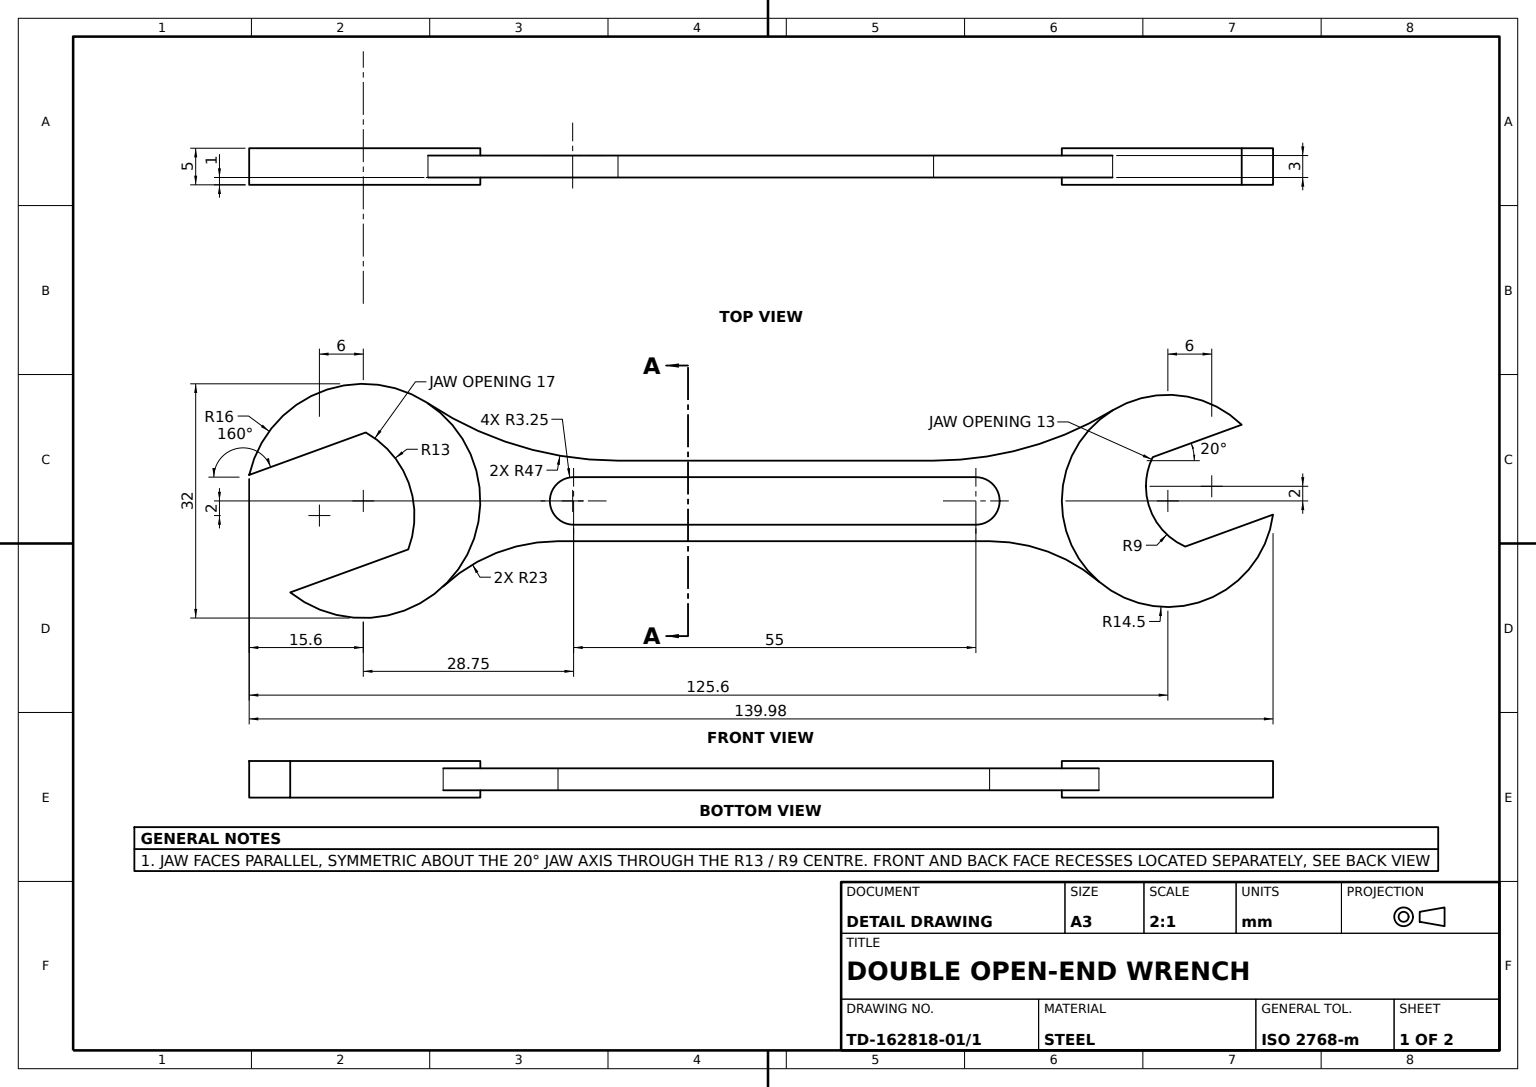
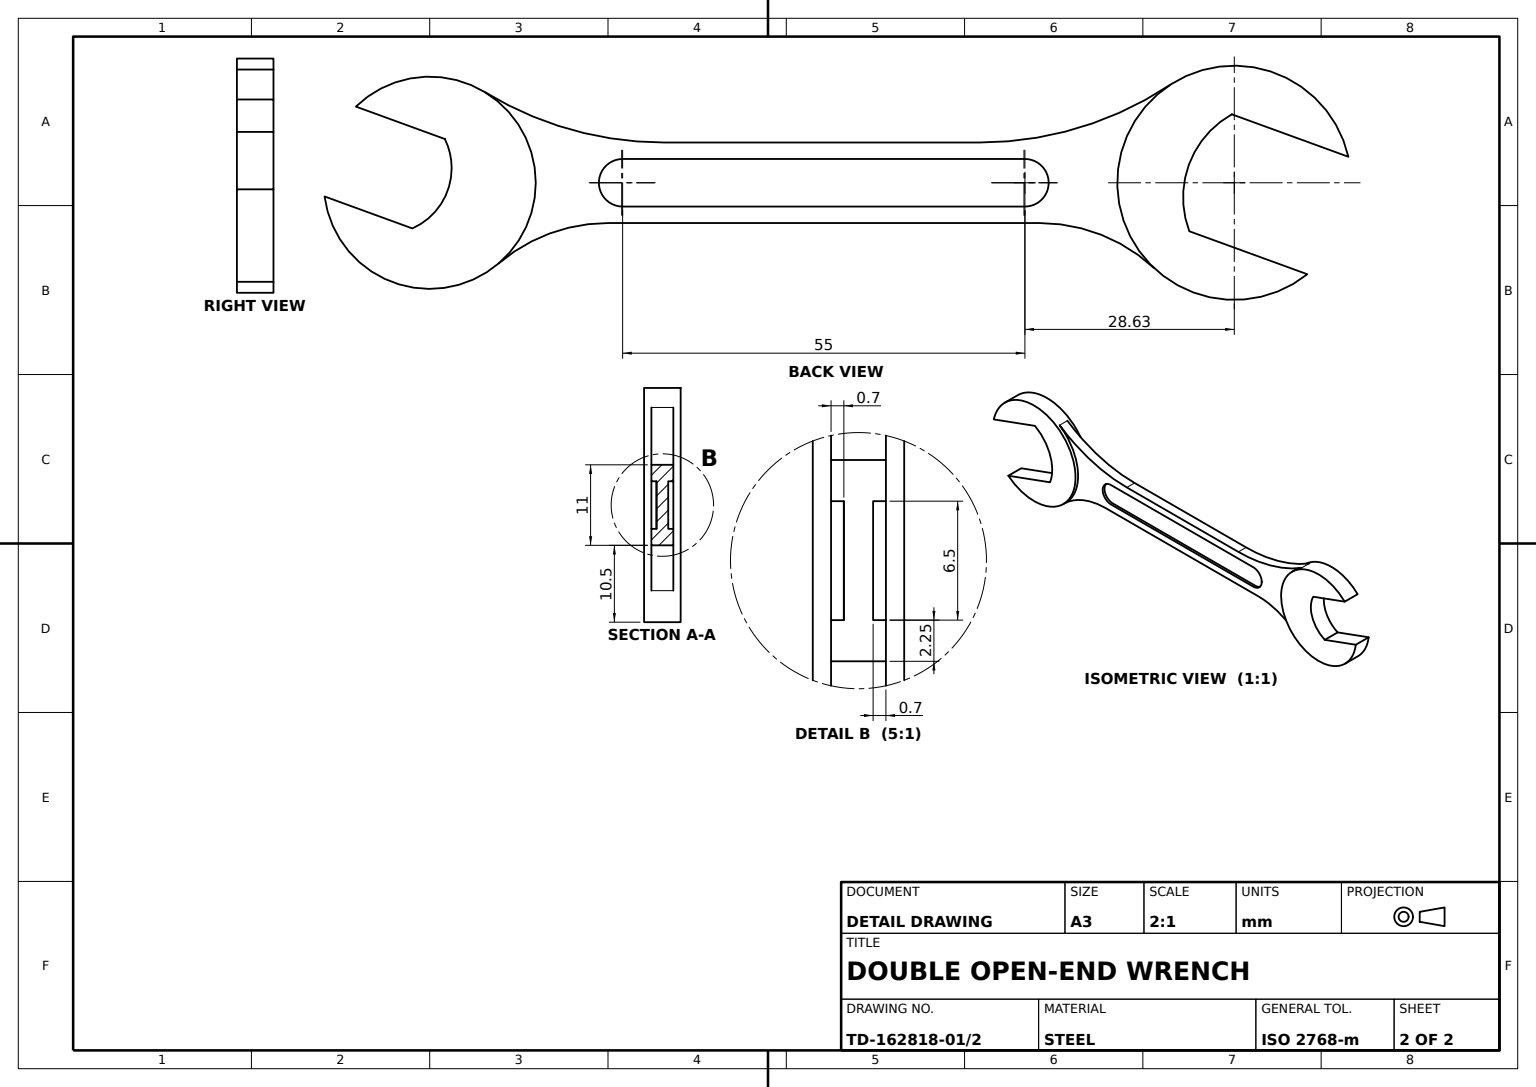
from build123d import *

# Parameters (mm, degrees)
SPANNER_BODY_3MM_DEPTH          = 3
HEAD_PAD_13_SIDE_A_DEPTH        = 1
HEAD_START                      = 1
HEAD_PAD_13_SIDE_B_DEPTH        = 1
HEAD_PAD_9_SIDE_A_DEPTH         = 1
HEAD_PAD_9_SIDE_B_DEPTH         = 1
HANDLE_SLOT_SIDE_A_55X6_5_DEPTH = 0.7
HANDLE_SLOT_SIDE_B_55X6_5_DEPTH = 0.7


with BuildPart() as part:
    # Spanner Profile Sketch → Spanner Body 3mm (new body)
    with BuildSketch(Plane.XY):
        with BuildLine():
            ThreePointArc((0.335793671, 9.351551373), (4.669621374, 5.426922629), (6.845232579, 0))
            Line((6.845232579, 0), (107.225035612, 0))
            ThreePointArc((107.225035612, 0), (107.061451957, 3.049932803), (107.927329677, 5.978943813))
            Line((107.927329677, 5.978943813), (120.095812241, 10.407909262))
            ThreePointArc((120.095812241, 10.407909262), (111.608728128, 14.410482081), (102.447920261, 12.37804878))
            ThreePointArc((102.447920261, 12.37804878), (90.682307093, 7.25217294), (77.968765244, 5.5))
            Line((77.968765244, 5.5), (34.824560299, 5.5))
            ThreePointArc((34.824560299, 5.5), (21.256828973, 7.500925935), (8.844332774, 13.333333333))
            ThreePointArc((8.844332774, 13.333333333), (-5.944434547, 14.854753378), (-15.600963823, 3.551046014))
            Line((-15.600963823, 3.551046014), (0.335793671, 9.351551373))
        make_face()
        with BuildLine():
            Line((107.225035612, 0), (6.845232579, 0))
            ThreePointArc((6.845232579, 0), (6.928993977, -3.356876833), (6.150136107, -6.623223181))
            Line((6.150136107, -6.623223181), (-9.990209349, -12.497828498))
            ThreePointArc((-9.990209349, -12.497828498), (0.615850097, -15.988143377), (10.921993446, -11.692307692))
            ThreePointArc((10.921993446, -11.692307692), (18.183666088, -7.104008283), (26.622359024, -5.5))
            Line((26.622359024, -5.5), (85.627884786, -5.5))
            ThreePointArc((85.627884786, -5.5), (93.595318501, -6.924087505), (100.576115451, -11.02))
            ThreePointArc((100.576115451, -11.02), (115.204003038, -13.533970311), (124.379255248, -1.867356026))
            Line((124.379255248, -1.867356026), (112.37359154, -6.237060258))
            ThreePointArc((112.37359154, -6.237060258), (109.059269326, -3.729420365), (107.225035612, 0))
        make_face()
    extrude(amount=SPANNER_BODY_3MM_DEPTH)

    # Head Pad 13 Side A Sketch → Head Pad 13 Side A (add)
    with BuildSketch(Plane.XY.offset(3)):
        with BuildLine():
            Line((-15.600963823, 3.551046014), (0.335793671, 9.351551373))
            ThreePointArc((0.335793671, 9.351551373), (6.21600407, 2.446261863), (6.150136107, -6.623223181))
            Line((6.150136107, -6.623223181), (-9.990209349, -12.497828498))
            ThreePointArc((-9.990209349, -12.497828498), (15.10359657, 5.280281303), (-15.600963823, 3.551046014))
        make_face()
    extrude(amount=HEAD_PAD_13_SIDE_A_DEPTH)

    # Head Pad 13 Side B Sketch → Head Pad 13 Side B (add)
    with BuildSketch(Plane(origin=(0, 0, 0), x_dir=(-1, 0, 0), z_dir=(0, 0, -1)).offset(HEAD_START)):
        with BuildLine():
            Line((-0.335793671, 9.351551373), (15.600963823, 3.551046014))
            ThreePointArc((15.600963823, 3.551046014), (-15.10359657, 5.280281303), (9.990209349, -12.497828498))
            Line((9.990209349, -12.497828498), (-6.150136107, -6.623223181))
            ThreePointArc((-6.150136107, -6.623223181), (-6.21600407, 2.446261863), (-0.335793671, 9.351551373))
        make_face()
    extrude(amount=-HEAD_PAD_13_SIDE_B_DEPTH)

    # Head Pad 9 Side A Sketch → Head Pad 9 Side A (add)
    with BuildSketch(Plane(origin=(0, 0, 0), x_dir=(-1, 0, 0), z_dir=(0, 0, -1)).offset(HEAD_START)):
        with BuildLine():
            Line((-107.927329677, 5.978943813), (-120.095812241, 10.407909262))
            ThreePointArc((-120.095812241, 10.407909262), (-96.309573907, -4.777262123), (-124.379255248, -1.867356026))
            Line((-124.379255248, -1.867356026), (-112.37359154, -6.237060258))
            ThreePointArc((-112.37359154, -6.237060258), (-107.542766412, -1.07818129), (-107.927329677, 5.978943813))
        make_face()
    extrude(amount=-HEAD_PAD_9_SIDE_A_DEPTH)

    # Head Pad 9 Side B Sketch → Head Pad 9 Side B (add)
    with BuildSketch(Plane.XY.offset(3)):
        with BuildLine():
            Line((107.927329677, 5.978943813), (120.095812241, 10.407909262))
            ThreePointArc((120.095812241, 10.407909262), (96.309573907, -4.777262123), (124.379255248, -1.867356026))
            Line((124.379255248, -1.867356026), (112.37359154, -6.237060258))
            ThreePointArc((112.37359154, -6.237060258), (107.542766412, -1.07818129), (107.927329677, 5.978943813))
        make_face()
    extrude(amount=HEAD_PAD_9_SIDE_B_DEPTH)

    # Handle Slot Side A Sketch → Handle Slot Side A 55x6.5 (cut)
    with BuildSketch(Plane.XY.offset(3)):
        with BuildLine():
            Line((28.768116085, 3.25), (83.753668591, 3.25))
            ThreePointArc((83.753668591, 3.25), (87.003668591, 0), (83.753668591, -3.25))
            Line((83.753668591, -3.25), (28.753668591, -3.250032112))
            ThreePointArc((28.753668591, -3.250032112), (25.503644507, 0.007223765), (28.768116085, 3.25))
        make_face()
    extrude(amount=-HANDLE_SLOT_SIDE_A_55X6_5_DEPTH, mode=Mode.SUBTRACT)

    # Handle Slot Side B Sketch → Handle Slot Side B 55x6.5 (cut)
    with BuildSketch(Plane(origin=(0, 0, 0), x_dir=(-1, 0, 0), z_dir=(0, 0, -1))):
        with BuildLine():
            Line((-83.625121905, 3.25), (-28.625121905, 3.25))
            ThreePointArc((-28.625121905, 3.25), (-25.375121905, 0), (-28.625121905, -3.25))
            Line((-28.625121905, -3.25), (-83.625121905, -3.25))
            ThreePointArc((-83.625121905, -3.25), (-86.875121905, 0), (-83.625121905, 3.25))
        make_face()
    extrude(amount=-HANDLE_SLOT_SIDE_B_55X6_5_DEPTH, mode=Mode.SUBTRACT)


solid = part.part
